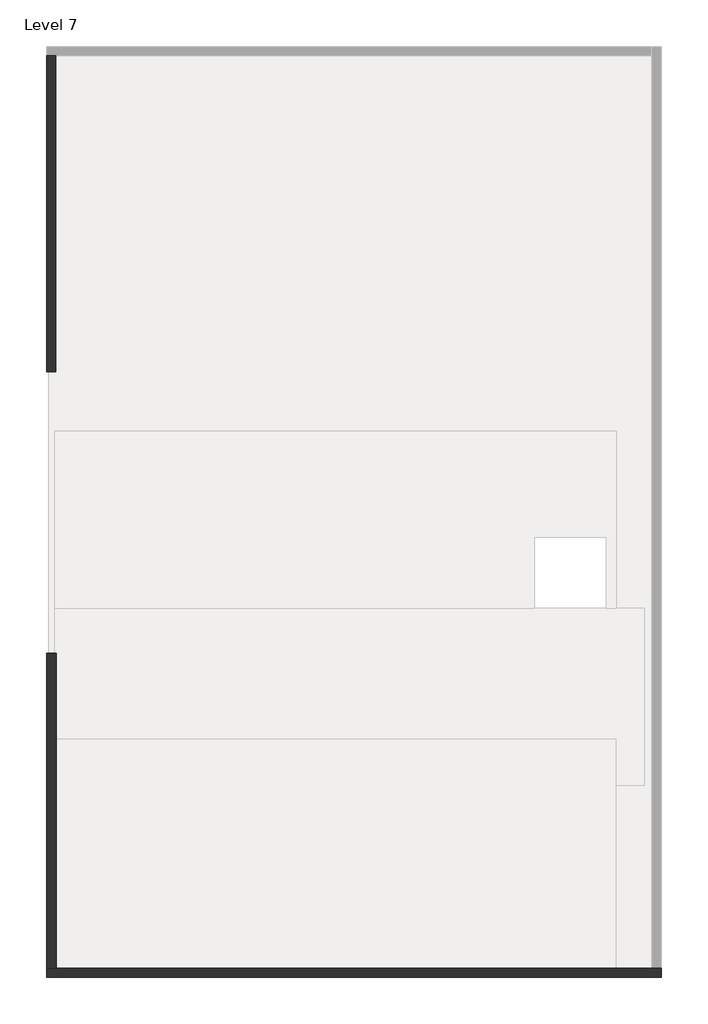
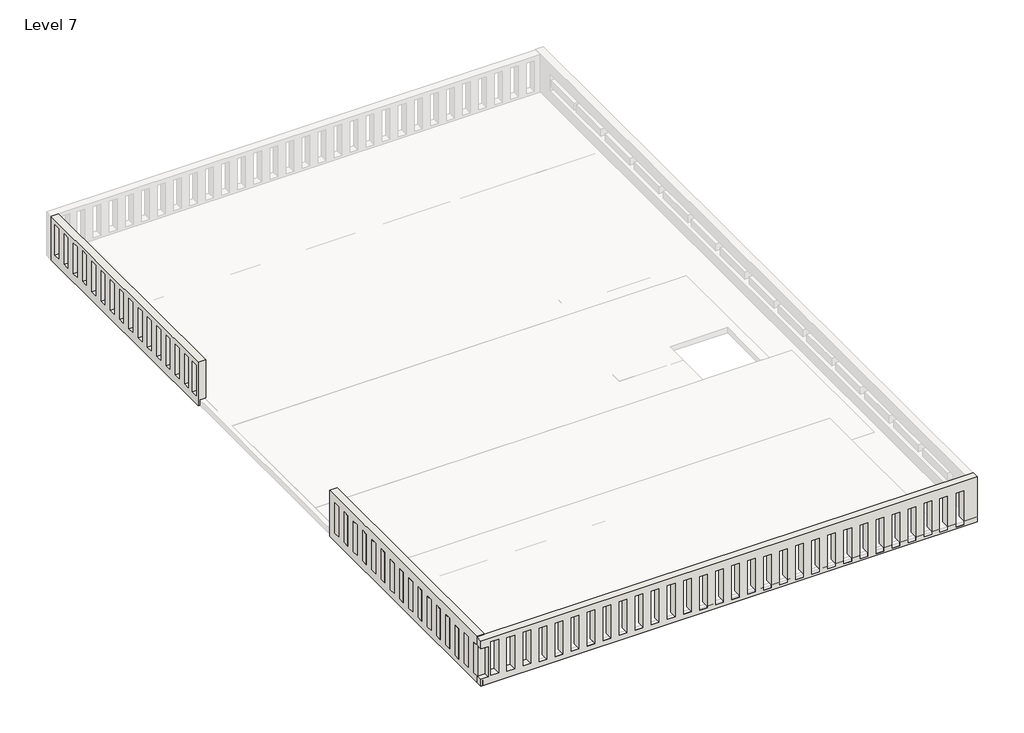
# One storey, part 1 of 2: 3 walls.
"""IFC4 building model written with IfcOpenShell, lengths in millimetres."""

from ifc_helpers import new_model, si_unit, origin, place, context, project, spatial, faceted_brep, element, save

model = new_model("IFC4")

# Units and contexts
model_context = context("Model", 3, world=origin())
ifc_project = project(units=[si_unit("LENGTHUNIT", "METRE", prefix="MILLI")], contexts=[model_context])

# Site, building, storey
site = spatial("IfcSite", under=ifc_project)
building = spatial("IfcBuilding", under=site)
storey = spatial("IfcBuildingStorey", under=building, Name="Level 7", Elevation=18288.0)

# Walls
placement = place(None, origin())
element("IfcWall", 1, ObjectType="Generic - 9\" w", at=placement, inside=storey, context=model_context, shape_type="Brep", body=[
    faceted_brep([(6853.7890963, -10500.4694836, 18288.0), (6650.5890963, -10500.4694836, 18288.0), (-6296.5895774, -10500.4694836, 18288.0), (-6499.7895774, -10500.4694836, 18288.0), (-6499.7895774, -10500.4694836, 18487.795072), (-6303.4109037, -10500.4694836, 18487.795072), (-6303.4109037, -10500.4694836, 19351.395072), (-6499.7895774, -10500.4694836, 19351.395072), (-6499.7895774, -10500.4694836, 19568.7926921), (6853.7890963, -10500.4694836, 19568.7926921), (6853.7890963, -10500.4694836, 19542.6572919), (-6026.0013636, -10500.4694836, 19465.6802167), (-6229.2013636, -10500.4694836, 19465.6802167), (-6229.2013636, -10500.4694836, 18509.4623037), (-6026.0013636, -10500.4694836, 18509.4623037), (-5595.844493, -10500.4694836, 19428.046367), (-5799.044493, -10500.4694836, 19428.046367), (-5799.044493, -10500.4694836, 18471.8284539), (-5595.844493, -10500.4694836, 18471.8284539), (-5164.044493, -10500.4694836, 19428.046367), (-5367.244493, -10500.4694836, 19428.046367), (-5367.244493, -10500.4694836, 18471.8284539), (-5164.044493, -10500.4694836, 18471.8284539), (-4733.8876223, -10500.4694836, 19390.4125173), (-4937.0876223, -10500.4694836, 19390.4125173), (-4937.0876223, -10500.4694836, 18434.1946042), (-4733.8876223, -10500.4694836, 18434.1946042), (-4302.0876223, -10500.4694836, 19390.4125173), (-4505.2876223, -10500.4694836, 19390.4125173), (-4505.2876223, -10500.4694836, 18434.1946042), (-4302.0876223, -10500.4694836, 18434.1946042), (-3870.2876223, -10500.4694836, 19390.4125173), (-4073.4876223, -10500.4694836, 19390.4125173), (-4073.4876223, -10500.4694836, 18434.1946042), (-3870.2876223, -10500.4694836, 18434.1946042), (-3438.4876223, -10500.4694836, 19390.4125173), (-3641.6876223, -10500.4694836, 19390.4125173), (-3641.6876223, -10500.4694836, 18434.1946042), (-3438.4876223, -10500.4694836, 18434.1946042), (-3006.6876223, -10500.4694836, 19390.4125173), (-3209.8876223, -10500.4694836, 19390.4125173), (-3209.8876223, -10500.4694836, 18434.1946042), (-3006.6876223, -10500.4694836, 18434.1946042), (-2574.8876223, -10500.4694836, 19390.4125173), (-2778.0876223, -10500.4694836, 19390.4125173), (-2778.0876223, -10500.4694836, 18434.1946042), (-2574.8876223, -10500.4694836, 18434.1946042), (-2143.0876223, -10500.4694836, 19390.4125173), (-2346.2876223, -10500.4694836, 19390.4125173), (-2346.2876223, -10500.4694836, 18434.1946042), (-2143.0876223, -10500.4694836, 18434.1946042), (-1711.2876223, -10500.4694836, 19390.4125173), (-1914.4876223, -10500.4694836, 19390.4125173), (-1914.4876223, -10500.4694836, 18434.1946042), (-1711.2876223, -10500.4694836, 18434.1946042), (-1279.4876223, -10500.4694836, 19390.4125173), (-1482.6876223, -10500.4694836, 19390.4125173), (-1482.6876223, -10500.4694836, 18434.1946042), (-1279.4876223, -10500.4694836, 18434.1946042), (-847.6876223, -10500.4694836, 19390.4125173), (-1050.8876223, -10500.4694836, 19390.4125173), (-1050.8876223, -10500.4694836, 18434.1946042), (-847.6876223, -10500.4694836, 18434.1946042), (-417.5307517, -10500.4694836, 19352.7786675), (-620.7307517, -10500.4694836, 19352.7786675), (-620.7307517, -10500.4694836, 18396.5607545), (-417.5307517, -10500.4694836, 18396.5607545), (14.2692483, -10500.4694836, 19352.7786675), (-188.9307517, -10500.4694836, 19352.7786675), (-188.9307517, -10500.4694836, 18396.5607545), (14.2692483, -10500.4694836, 18396.5607545), (446.0692483, -10500.4694836, 19352.7786675), (242.8692483, -10500.4694836, 19352.7786675), (242.8692483, -10500.4694836, 18396.5607545), (446.0692483, -10500.4694836, 18396.5607545), (877.8692483, -10500.4694836, 19352.7786675), (674.6692483, -10500.4694836, 19352.7786675), (674.6692483, -10500.4694836, 18396.5607545), (877.8692483, -10500.4694836, 18396.5607545), (1308.0261189, -10500.4694836, 19315.1448178), (1104.8261189, -10500.4694836, 19315.1448178), (1104.8261189, -10500.4694836, 18358.9269048), (1308.0261189, -10500.4694836, 18358.9269048), (1739.8261189, -10500.4694836, 19315.1448178), (1536.6261189, -10500.4694836, 19315.1448178), (1536.6261189, -10500.4694836, 18358.9269048), (1739.8261189, -10500.4694836, 18358.9269048), (2171.6261189, -10500.4694836, 19315.1448178), (1968.4261189, -10500.4694836, 19315.1448178), (1968.4261189, -10500.4694836, 18358.9269048), (2171.6261189, -10500.4694836, 18358.9269048), (2603.4261189, -10500.4694836, 19315.1448178), (2400.2261189, -10500.4694836, 19315.1448178), (2400.2261189, -10500.4694836, 18358.9269048), (2603.4261189, -10500.4694836, 18358.9269048), (3035.2261189, -10500.4694836, 19315.1448178), (2832.0261189, -10500.4694836, 19315.1448178), (2832.0261189, -10500.4694836, 18358.9269048), (3035.2261189, -10500.4694836, 18358.9269048), (3467.0261189, -10500.4694836, 19315.1448178), (3263.8261189, -10500.4694836, 19315.1448178), (3263.8261189, -10500.4694836, 18358.9269048), (3467.0261189, -10500.4694836, 18358.9269048), (3898.5630781, -10500.4694836, 19300.0752152), (3695.3630781, -10500.4694836, 19300.0752152), (3695.3630781, -10500.4694836, 18343.8573021), (3898.5630781, -10500.4694836, 18343.8573021), (4330.3630781, -10500.4694836, 19300.0752152), (4127.1630781, -10500.4694836, 19300.0752152), (4127.1630781, -10500.4694836, 18343.8573021), (4330.3630781, -10500.4694836, 18343.8573021), (4762.1630781, -10500.4694836, 19300.0752152), (4558.9630781, -10500.4694836, 19300.0752152), (4558.9630781, -10500.4694836, 18343.8573021), (4762.1630781, -10500.4694836, 18343.8573021), (5193.9630781, -10500.4694836, 19300.0752152), (4990.7630781, -10500.4694836, 19300.0752152), (4990.7630781, -10500.4694836, 18343.8573021), (5193.9630781, -10500.4694836, 18343.8573021), (6044.4430536, -10500.4694836, 19300.0752152), (5841.2430536, -10500.4694836, 19300.0752152), (5841.2430536, -10500.4694836, 18343.8573021), (6044.4430536, -10500.4694836, 18343.8573021), (6485.4890963, -10500.4694836, 19300.0752152), (6282.2890963, -10500.4694836, 19300.0752152), (6282.2890963, -10500.4694836, 18343.8573021), (6485.4890963, -10500.4694836, 18343.8573021), (5625.1713112, -10500.4694836, 19322.6738811), (5421.9713112, -10500.4694836, 19322.6738811), (5421.9713112, -10500.4694836, 18366.455968), (5625.1713112, -10500.4694836, 18366.455968), (6853.7890963, -10703.6694836, 18288.0), (6853.7890963, -10703.6694836, 19568.7926921), (-6499.7895774, -10703.6694836, 19568.7926921), (-6499.7895774, -10703.6694836, 19351.395072), (-6303.4109037, -10703.6694836, 19351.395072), (-6303.4109037, -10703.6694836, 18487.795072), (-6499.7895774, -10703.6694836, 18487.795072), (-6499.7895774, -10703.6694836, 18288.0), (-6026.0013636, -10703.6694836, 19465.6802167), (-6026.0013636, -10703.6694836, 18509.4623037), (-6229.2013636, -10703.6694836, 18509.4623037), (-6229.2013636, -10703.6694836, 19465.6802167), (-5595.844493, -10703.6694836, 19428.046367), (-5595.844493, -10703.6694836, 18471.8284539), (-5799.044493, -10703.6694836, 18471.8284539), (-5799.044493, -10703.6694836, 19428.046367), (-5164.044493, -10703.6694836, 19428.046367), (-5164.044493, -10703.6694836, 18471.8284539), (-5367.244493, -10703.6694836, 18471.8284539), (-5367.244493, -10703.6694836, 19428.046367), (-4733.8876223, -10703.6694836, 19390.4125173), (-4733.8876223, -10703.6694836, 18434.1946042), (-4937.0876223, -10703.6694836, 18434.1946042), (-4937.0876223, -10703.6694836, 19390.4125173), (-4302.0876223, -10703.6694836, 19390.4125173), (-4302.0876223, -10703.6694836, 18434.1946042), (-4505.2876223, -10703.6694836, 18434.1946042), (-4505.2876223, -10703.6694836, 19390.4125173), (-3870.2876223, -10703.6694836, 19390.4125173), (-3870.2876223, -10703.6694836, 18434.1946042), (-4073.4876223, -10703.6694836, 18434.1946042), (-4073.4876223, -10703.6694836, 19390.4125173), (-3438.4876223, -10703.6694836, 19390.4125173), (-3438.4876223, -10703.6694836, 18434.1946042), (-3641.6876223, -10703.6694836, 18434.1946042), (-3641.6876223, -10703.6694836, 19390.4125173), (-3006.6876223, -10703.6694836, 19390.4125173), (-3006.6876223, -10703.6694836, 18434.1946042), (-3209.8876223, -10703.6694836, 18434.1946042), (-3209.8876223, -10703.6694836, 19390.4125173), (-2574.8876223, -10703.6694836, 19390.4125173), (-2574.8876223, -10703.6694836, 18434.1946042), (-2778.0876223, -10703.6694836, 18434.1946042), (-2778.0876223, -10703.6694836, 19390.4125173), (-2143.0876223, -10703.6694836, 19390.4125173), (-2143.0876223, -10703.6694836, 18434.1946042), (-2346.2876223, -10703.6694836, 18434.1946042), (-2346.2876223, -10703.6694836, 19390.4125173), (-1711.2876223, -10703.6694836, 19390.4125173), (-1711.2876223, -10703.6694836, 18434.1946042), (-1914.4876223, -10703.6694836, 18434.1946042), (-1914.4876223, -10703.6694836, 19390.4125173), (-1279.4876223, -10703.6694836, 19390.4125173), (-1279.4876223, -10703.6694836, 18434.1946042), (-1482.6876223, -10703.6694836, 18434.1946042), (-1482.6876223, -10703.6694836, 19390.4125173), (-847.6876223, -10703.6694836, 19390.4125173), (-847.6876223, -10703.6694836, 18434.1946042), (-1050.8876223, -10703.6694836, 18434.1946042), (-1050.8876223, -10703.6694836, 19390.4125173), (-417.5307517, -10703.6694836, 19352.7786675), (-417.5307517, -10703.6694836, 18396.5607545), (-620.7307517, -10703.6694836, 18396.5607545), (-620.7307517, -10703.6694836, 19352.7786675), (14.2692483, -10703.6694836, 19352.7786675), (14.2692483, -10703.6694836, 18396.5607545), (-188.9307517, -10703.6694836, 18396.5607545), (-188.9307517, -10703.6694836, 19352.7786675), (446.0692483, -10703.6694836, 19352.7786675), (446.0692483, -10703.6694836, 18396.5607545), (242.8692483, -10703.6694836, 18396.5607545), (242.8692483, -10703.6694836, 19352.7786675), (877.8692483, -10703.6694836, 19352.7786675), (877.8692483, -10703.6694836, 18396.5607545), (674.6692483, -10703.6694836, 18396.5607545), (674.6692483, -10703.6694836, 19352.7786675), (1308.0261189, -10703.6694836, 19315.1448178), (1308.0261189, -10703.6694836, 18358.9269048), (1104.8261189, -10703.6694836, 18358.9269048), (1104.8261189, -10703.6694836, 19315.1448178), (1739.8261189, -10703.6694836, 19315.1448178), (1739.8261189, -10703.6694836, 18358.9269048), (1536.6261189, -10703.6694836, 18358.9269048), (1536.6261189, -10703.6694836, 19315.1448178), (2171.6261189, -10703.6694836, 19315.1448178), (2171.6261189, -10703.6694836, 18358.9269048), (1968.4261189, -10703.6694836, 18358.9269048), (1968.4261189, -10703.6694836, 19315.1448178), (2603.4261189, -10703.6694836, 19315.1448178), (2603.4261189, -10703.6694836, 18358.9269048), (2400.2261189, -10703.6694836, 18358.9269048), (2400.2261189, -10703.6694836, 19315.1448178), (3035.2261189, -10703.6694836, 19315.1448178), (3035.2261189, -10703.6694836, 18358.9269048), (2832.0261189, -10703.6694836, 18358.9269048), (2832.0261189, -10703.6694836, 19315.1448178), (3467.0261189, -10703.6694836, 19315.1448178), (3467.0261189, -10703.6694836, 18358.9269048), (3263.8261189, -10703.6694836, 18358.9269048), (3263.8261189, -10703.6694836, 19315.1448178), (3898.5630781, -10703.6694836, 19300.0752152), (3898.5630781, -10703.6694836, 18343.8573021), (3695.3630781, -10703.6694836, 18343.8573021), (3695.3630781, -10703.6694836, 19300.0752152), (4330.3630781, -10703.6694836, 19300.0752152), (4330.3630781, -10703.6694836, 18343.8573021), (4127.1630781, -10703.6694836, 18343.8573021), (4127.1630781, -10703.6694836, 19300.0752152), (4762.1630781, -10703.6694836, 19300.0752152), (4762.1630781, -10703.6694836, 18343.8573021), (4558.9630781, -10703.6694836, 18343.8573021), (4558.9630781, -10703.6694836, 19300.0752152), (5193.9630781, -10703.6694836, 19300.0752152), (5193.9630781, -10703.6694836, 18343.8573021), (4990.7630781, -10703.6694836, 18343.8573021), (4990.7630781, -10703.6694836, 19300.0752152), (6044.4430536, -10703.6694836, 19300.0752152), (6044.4430536, -10703.6694836, 18343.8573021), (5841.2430536, -10703.6694836, 18343.8573021), (5841.2430536, -10703.6694836, 19300.0752152), (6485.4890963, -10703.6694836, 19300.0752152), (6485.4890963, -10703.6694836, 18343.8573021), (6282.2890963, -10703.6694836, 18343.8573021), (6282.2890963, -10703.6694836, 19300.0752152), (5625.1713112, -10703.6694836, 19322.6738811), (5625.1713112, -10703.6694836, 18366.455968), (5421.9713112, -10703.6694836, 18366.455968), (5421.9713112, -10703.6694836, 19322.6738811), (-6303.4109037, -10557.1743868, 18487.795072), (-6303.4109037, -10557.1743868, 19351.395072)], [[[0, 1, 2, 3, 4, 5, 6, 7, 8, 9, 10], [11, 12, 13, 14], [15, 16, 17, 18], [19, 20, 21, 22], [23, 24, 25, 26], [27, 28, 29, 30], [31, 32, 33, 34], [35, 36, 37, 38], [39, 40, 41, 42], [43, 44, 45, 46], [47, 48, 49, 50], [51, 52, 53, 54], [55, 56, 57, 58], [59, 60, 61, 62], [63, 64, 65, 66], [67, 68, 69, 70], [71, 72, 73, 74], [75, 76, 77, 78], [79, 80, 81, 82], [83, 84, 85, 86], [87, 88, 89, 90], [91, 92, 93, 94], [95, 96, 97, 98], [99, 100, 101, 102], [103, 104, 105, 106], [107, 108, 109, 110], [111, 112, 113, 114], [115, 116, 117, 118], [119, 120, 121, 122], [123, 124, 125, 126], [127, 128, 129, 130]], [[131, 132, 133, 134, 135, 136, 137, 138], [139, 140, 141, 142], [143, 144, 145, 146], [147, 148, 149, 150], [151, 152, 153, 154], [155, 156, 157, 158], [159, 160, 161, 162], [163, 164, 165, 166], [167, 168, 169, 170], [171, 172, 173, 174], [175, 176, 177, 178], [179, 180, 181, 182], [183, 184, 185, 186], [187, 188, 189, 190], [191, 192, 193, 194], [195, 196, 197, 198], [199, 200, 201, 202], [203, 204, 205, 206], [207, 208, 209, 210], [211, 212, 213, 214], [215, 216, 217, 218], [219, 220, 221, 222], [223, 224, 225, 226], [227, 228, 229, 230], [231, 232, 233, 234], [235, 236, 237, 238], [239, 240, 241, 242], [243, 244, 245, 246], [247, 248, 249, 250], [251, 252, 253, 254], [255, 256, 257, 258]], [[0, 10, 9, 132, 131]], [[4, 3, 138, 137]], [[6, 5, 259, 136, 135, 260]], [[8, 7, 134, 133]], [[3, 2, 1, 0, 131, 138]], [[9, 8, 133, 132]], [[136, 259, 5, 4, 137]], [[134, 7, 6, 260, 135]], [[12, 11, 139, 142]], [[13, 12, 142, 141]], [[14, 13, 141, 140]], [[11, 14, 140, 139]], [[16, 15, 143, 146]], [[17, 16, 146, 145]], [[18, 17, 145, 144]], [[15, 18, 144, 143]], [[20, 19, 147, 150]], [[21, 20, 150, 149]], [[22, 21, 149, 148]], [[19, 22, 148, 147]], [[24, 23, 151, 154]], [[25, 24, 154, 153]], [[26, 25, 153, 152]], [[23, 26, 152, 151]], [[28, 27, 155, 158]], [[29, 28, 158, 157]], [[30, 29, 157, 156]], [[27, 30, 156, 155]], [[32, 31, 159, 162]], [[33, 32, 162, 161]], [[34, 33, 161, 160]], [[31, 34, 160, 159]], [[36, 35, 163, 166]], [[37, 36, 166, 165]], [[38, 37, 165, 164]], [[35, 38, 164, 163]], [[40, 39, 167, 170]], [[41, 40, 170, 169]], [[42, 41, 169, 168]], [[39, 42, 168, 167]], [[44, 43, 171, 174]], [[45, 44, 174, 173]], [[46, 45, 173, 172]], [[43, 46, 172, 171]], [[48, 47, 175, 178]], [[49, 48, 178, 177]], [[50, 49, 177, 176]], [[47, 50, 176, 175]], [[52, 51, 179, 182]], [[53, 52, 182, 181]], [[54, 53, 181, 180]], [[51, 54, 180, 179]], [[56, 55, 183, 186]], [[57, 56, 186, 185]], [[58, 57, 185, 184]], [[55, 58, 184, 183]], [[60, 59, 187, 190]], [[61, 60, 190, 189]], [[62, 61, 189, 188]], [[59, 62, 188, 187]], [[64, 63, 191, 194]], [[65, 64, 194, 193]], [[66, 65, 193, 192]], [[63, 66, 192, 191]], [[68, 67, 195, 198]], [[69, 68, 198, 197]], [[70, 69, 197, 196]], [[67, 70, 196, 195]], [[72, 71, 199, 202]], [[73, 72, 202, 201]], [[74, 73, 201, 200]], [[71, 74, 200, 199]], [[76, 75, 203, 206]], [[77, 76, 206, 205]], [[78, 77, 205, 204]], [[75, 78, 204, 203]], [[80, 79, 207, 210]], [[81, 80, 210, 209]], [[82, 81, 209, 208]], [[79, 82, 208, 207]], [[84, 83, 211, 214]], [[85, 84, 214, 213]], [[86, 85, 213, 212]], [[83, 86, 212, 211]], [[88, 87, 215, 218]], [[89, 88, 218, 217]], [[90, 89, 217, 216]], [[87, 90, 216, 215]], [[92, 91, 219, 222]], [[93, 92, 222, 221]], [[94, 93, 221, 220]], [[91, 94, 220, 219]], [[96, 95, 223, 226]], [[97, 96, 226, 225]], [[98, 97, 225, 224]], [[95, 98, 224, 223]], [[100, 99, 227, 230]], [[101, 100, 230, 229]], [[102, 101, 229, 228]], [[99, 102, 228, 227]], [[104, 103, 231, 234]], [[105, 104, 234, 233]], [[106, 105, 233, 232]], [[103, 106, 232, 231]], [[108, 107, 235, 238]], [[109, 108, 238, 237]], [[110, 109, 237, 236]], [[107, 110, 236, 235]], [[112, 111, 239, 242]], [[113, 112, 242, 241]], [[114, 113, 241, 240]], [[111, 114, 240, 239]], [[116, 115, 243, 246]], [[117, 116, 246, 245]], [[118, 117, 245, 244]], [[115, 118, 244, 243]], [[120, 119, 247, 250]], [[121, 120, 250, 249]], [[122, 121, 249, 248]], [[119, 122, 248, 247]], [[124, 123, 251, 254]], [[125, 124, 254, 253]], [[126, 125, 253, 252]], [[123, 126, 252, 251]], [[128, 127, 255, 258]], [[129, 128, 258, 257]], [[130, 129, 257, 256]], [[127, 130, 256, 255]]]),
])
element("IfcWall", 2, ObjectType="Generic - 9\" w", at=placement, inside=storey, context=model_context, shape_type="Brep", body=[
    faceted_brep([(-6506.6109037, 9313.3962251, 18288.0), (-6506.6109037, 2455.3962251, 18288.0), (-6506.6109037, 2455.3962251, 19520.2498043), (-6506.6109037, 9313.3962251, 19520.2498043), (-6506.6109037, 8952.0816143, 19389.0289217), (-6506.6109037, 8952.0816143, 18525.4289217), (-6506.6109037, 9129.8816143, 18525.4289217), (-6506.6109037, 9129.8816143, 19389.0289217), (-6506.6109037, 8520.2816143, 19389.0289217), (-6506.6109037, 8520.2816143, 18525.4289217), (-6506.6109037, 8698.0816143, 18525.4289217), (-6506.6109037, 8698.0816143, 19389.0289217), (-6506.6109037, 8088.4816143, 19389.0289217), (-6506.6109037, 8088.4816143, 18525.4289217), (-6506.6109037, 8266.2816143, 18525.4289217), (-6506.6109037, 8266.2816143, 19389.0289217), (-6506.6109037, 7658.3247436, 19426.6627714), (-6506.6109037, 7658.3247436, 18563.0627714), (-6506.6109037, 7836.1247436, 18563.0627714), (-6506.6109037, 7836.1247436, 19426.6627714), (-6506.6109037, 7228.167873, 19389.0289217), (-6506.6109037, 7228.167873, 18525.4289217), (-6506.6109037, 7405.967873, 18525.4289217), (-6506.6109037, 7405.967873, 19389.0289217), (-6506.6109037, 6796.367873, 19389.0289217), (-6506.6109037, 6796.367873, 18525.4289217), (-6506.6109037, 6974.167873, 18525.4289217), (-6506.6109037, 6974.167873, 19389.0289217), (-6506.6109037, 6364.567873, 19389.0289217), (-6506.6109037, 6364.567873, 18525.4289217), (-6506.6109037, 6542.367873, 18525.4289217), (-6506.6109037, 6542.367873, 19389.0289217), (-6506.6109037, 5932.767873, 19389.0289217), (-6506.6109037, 5932.767873, 18525.4289217), (-6506.6109037, 6110.567873, 18525.4289217), (-6506.6109037, 6110.567873, 19389.0289217), (-6506.6109037, 5500.967873, 19389.0289217), (-6506.6109037, 5500.967873, 18525.4289217), (-6506.6109037, 5678.767873, 18525.4289217), (-6506.6109037, 5678.767873, 19389.0289217), (-6506.6109037, 5069.167873, 19389.0289217), (-6506.6109037, 5069.167873, 18525.4289217), (-6506.6109037, 5246.967873, 18525.4289217), (-6506.6109037, 5246.967873, 19389.0289217), (-6506.6109037, 4637.367873, 19389.0289217), (-6506.6109037, 4637.367873, 18525.4289217), (-6506.6109037, 4815.167873, 18525.4289217), (-6506.6109037, 4815.167873, 19389.0289217), (-6506.6109037, 4205.567873, 19389.0289217), (-6506.6109037, 4205.567873, 18525.4289217), (-6506.6109037, 4383.367873, 18525.4289217), (-6506.6109037, 4383.367873, 19389.0289217), (-6506.6109037, 3773.767873, 19389.0289217), (-6506.6109037, 3773.767873, 18525.4289217), (-6506.6109037, 3951.567873, 18525.4289217), (-6506.6109037, 3951.567873, 19389.0289217), (-6506.6109037, 3341.967873, 19389.0289217), (-6506.6109037, 3341.967873, 18525.4289217), (-6506.6109037, 3519.767873, 18525.4289217), (-6506.6109037, 3519.767873, 19389.0289217), (-6506.6109037, 2910.167873, 19389.0289217), (-6506.6109037, 2910.167873, 18525.4289217), (-6506.6109037, 3087.967873, 18525.4289217), (-6506.6109037, 3087.967873, 19389.0289217), (-6506.6109037, 2544.2962251, 19389.0289217), (-6506.6109037, 2544.2962251, 18525.4289217), (-6506.6109037, 2722.0962251, 18525.4289217), (-6506.6109037, 2722.0962251, 19389.0289217), (-6303.4109037, 9313.3962251, 18288.0), (-6303.4109037, 9313.3962251, 19520.2498043), (-6303.4109037, 2455.3962251, 19520.2498043), (-6303.4109037, 2455.3962251, 18288.0), (-6303.4109037, 8952.0816143, 19389.0289217), (-6303.4109037, 9129.8816143, 19389.0289217), (-6303.4109037, 9129.8816143, 18525.4289217), (-6303.4109037, 8952.0816143, 18525.4289217), (-6303.4109037, 8520.2816143, 19389.0289217), (-6303.4109037, 8698.0816143, 19389.0289217), (-6303.4109037, 8698.0816143, 18525.4289217), (-6303.4109037, 8520.2816143, 18525.4289217), (-6303.4109037, 8088.4816143, 19389.0289217), (-6303.4109037, 8266.2816143, 19389.0289217), (-6303.4109037, 8266.2816143, 18525.4289217), (-6303.4109037, 8088.4816143, 18525.4289217), (-6303.4109037, 7658.3247436, 19426.6627714), (-6303.4109037, 7836.1247436, 19426.6627714), (-6303.4109037, 7836.1247436, 18563.0627714), (-6303.4109037, 7658.3247436, 18563.0627714), (-6303.4109037, 7228.167873, 19389.0289217), (-6303.4109037, 7405.967873, 19389.0289217), (-6303.4109037, 7405.967873, 18525.4289217), (-6303.4109037, 7228.167873, 18525.4289217), (-6303.4109037, 6796.367873, 19389.0289217), (-6303.4109037, 6974.167873, 19389.0289217), (-6303.4109037, 6974.167873, 18525.4289217), (-6303.4109037, 6796.367873, 18525.4289217), (-6303.4109037, 6364.567873, 19389.0289217), (-6303.4109037, 6542.367873, 19389.0289217), (-6303.4109037, 6542.367873, 18525.4289217), (-6303.4109037, 6364.567873, 18525.4289217), (-6303.4109037, 5932.767873, 19389.0289217), (-6303.4109037, 6110.567873, 19389.0289217), (-6303.4109037, 6110.567873, 18525.4289217), (-6303.4109037, 5932.767873, 18525.4289217), (-6303.4109037, 5500.967873, 19389.0289217), (-6303.4109037, 5678.767873, 19389.0289217), (-6303.4109037, 5678.767873, 18525.4289217), (-6303.4109037, 5500.967873, 18525.4289217), (-6303.4109037, 5069.167873, 19389.0289217), (-6303.4109037, 5246.967873, 19389.0289217), (-6303.4109037, 5246.967873, 18525.4289217), (-6303.4109037, 5069.167873, 18525.4289217), (-6303.4109037, 4637.367873, 19389.0289217), (-6303.4109037, 4815.167873, 19389.0289217), (-6303.4109037, 4815.167873, 18525.4289217), (-6303.4109037, 4637.367873, 18525.4289217), (-6303.4109037, 4205.567873, 19389.0289217), (-6303.4109037, 4383.367873, 19389.0289217), (-6303.4109037, 4383.367873, 18525.4289217), (-6303.4109037, 4205.567873, 18525.4289217), (-6303.4109037, 3773.767873, 19389.0289217), (-6303.4109037, 3951.567873, 19389.0289217), (-6303.4109037, 3951.567873, 18525.4289217), (-6303.4109037, 3773.767873, 18525.4289217), (-6303.4109037, 3341.967873, 19389.0289217), (-6303.4109037, 3519.767873, 19389.0289217), (-6303.4109037, 3519.767873, 18525.4289217), (-6303.4109037, 3341.967873, 18525.4289217), (-6303.4109037, 2910.167873, 19389.0289217), (-6303.4109037, 3087.967873, 19389.0289217), (-6303.4109037, 3087.967873, 18525.4289217), (-6303.4109037, 2910.167873, 18525.4289217), (-6303.4109037, 2544.2962251, 19389.0289217), (-6303.4109037, 2722.0962251, 19389.0289217), (-6303.4109037, 2722.0962251, 18525.4289217), (-6303.4109037, 2544.2962251, 18525.4289217)], [[[0, 1, 2, 3], [4, 5, 6, 7], [8, 9, 10, 11], [12, 13, 14, 15], [16, 17, 18, 19], [20, 21, 22, 23], [24, 25, 26, 27], [28, 29, 30, 31], [32, 33, 34, 35], [36, 37, 38, 39], [40, 41, 42, 43], [44, 45, 46, 47], [48, 49, 50, 51], [52, 53, 54, 55], [56, 57, 58, 59], [60, 61, 62, 63], [64, 65, 66, 67]], [[68, 69, 70, 71], [72, 73, 74, 75], [76, 77, 78, 79], [80, 81, 82, 83], [84, 85, 86, 87], [88, 89, 90, 91], [92, 93, 94, 95], [96, 97, 98, 99], [100, 101, 102, 103], [104, 105, 106, 107], [108, 109, 110, 111], [112, 113, 114, 115], [116, 117, 118, 119], [120, 121, 122, 123], [124, 125, 126, 127], [128, 129, 130, 131], [132, 133, 134, 135]], [[0, 3, 69, 68]], [[1, 0, 68, 71]], [[2, 1, 71, 70]], [[3, 2, 70, 69]], [[5, 4, 72, 75]], [[6, 5, 75, 74]], [[7, 6, 74, 73]], [[4, 7, 73, 72]], [[9, 8, 76, 79]], [[10, 9, 79, 78]], [[11, 10, 78, 77]], [[8, 11, 77, 76]], [[13, 12, 80, 83]], [[14, 13, 83, 82]], [[15, 14, 82, 81]], [[12, 15, 81, 80]], [[17, 16, 84, 87]], [[18, 17, 87, 86]], [[19, 18, 86, 85]], [[16, 19, 85, 84]], [[21, 20, 88, 91]], [[22, 21, 91, 90]], [[23, 22, 90, 89]], [[20, 23, 89, 88]], [[25, 24, 92, 95]], [[26, 25, 95, 94]], [[27, 26, 94, 93]], [[24, 27, 93, 92]], [[29, 28, 96, 99]], [[30, 29, 99, 98]], [[31, 30, 98, 97]], [[28, 31, 97, 96]], [[33, 32, 100, 103]], [[34, 33, 103, 102]], [[35, 34, 102, 101]], [[32, 35, 101, 100]], [[37, 36, 104, 107]], [[38, 37, 107, 106]], [[39, 38, 106, 105]], [[36, 39, 105, 104]], [[41, 40, 108, 111]], [[42, 41, 111, 110]], [[43, 42, 110, 109]], [[40, 43, 109, 108]], [[45, 44, 112, 115]], [[46, 45, 115, 114]], [[47, 46, 114, 113]], [[44, 47, 113, 112]], [[49, 48, 116, 119]], [[50, 49, 119, 118]], [[51, 50, 118, 117]], [[48, 51, 117, 116]], [[53, 52, 120, 123]], [[54, 53, 123, 122]], [[55, 54, 122, 121]], [[52, 55, 121, 120]], [[57, 56, 124, 127]], [[58, 57, 127, 126]], [[59, 58, 126, 125]], [[56, 59, 125, 124]], [[61, 60, 128, 131]], [[62, 61, 131, 130]], [[63, 62, 130, 129]], [[60, 63, 129, 128]], [[65, 64, 132, 135]], [[66, 65, 135, 134]], [[67, 66, 134, 133]], [[64, 67, 133, 132]]]),
    faceted_brep([(-6506.6109037, -4085.1037749, 19389.0289217), (-6506.6109037, -3907.3037749, 19389.0289217), (-6506.6109037, -3907.3037749, 18525.4289217), (-6506.6109037, -4085.1037749, 18525.4289217), (-6303.4109037, -4085.1037749, 19389.0289217), (-6303.4109037, -4085.1037749, 18525.4289217), (-6303.4109037, -3907.3037749, 18525.4289217), (-6303.4109037, -3907.3037749, 19389.0289217)], [[[0, 1, 2, 3]], [[4, 5, 6, 7]], [[1, 0, 4, 7]], [[2, 1, 7, 6]], [[3, 2, 6, 5]], [[0, 3, 5, 4]]]),
    faceted_brep([(-6506.6109037, -4516.9037749, 19389.0289217), (-6506.6109037, -4339.1037749, 19389.0289217), (-6506.6109037, -4339.1037749, 18525.4289217), (-6506.6109037, -4516.9037749, 18525.4289217), (-6303.4109037, -4516.9037749, 19389.0289217), (-6303.4109037, -4516.9037749, 18525.4289217), (-6303.4109037, -4339.1037749, 18525.4289217), (-6303.4109037, -4339.1037749, 19389.0289217)], [[[0, 1, 2, 3]], [[4, 5, 6, 7]], [[1, 0, 4, 7]], [[2, 1, 7, 6]], [[3, 2, 6, 5]], [[0, 3, 5, 4]]]),
    faceted_brep([(-6506.6109037, -4948.7037749, 19389.0289217), (-6506.6109037, -4770.9037749, 19389.0289217), (-6506.6109037, -4770.9037749, 18525.4289217), (-6506.6109037, -4948.7037749, 18525.4289217), (-6303.4109037, -4948.7037749, 19389.0289217), (-6303.4109037, -4948.7037749, 18525.4289217), (-6303.4109037, -4770.9037749, 18525.4289217), (-6303.4109037, -4770.9037749, 19389.0289217)], [[[0, 1, 2, 3]], [[4, 5, 6, 7]], [[1, 0, 4, 7]], [[2, 1, 7, 6]], [[3, 2, 6, 5]], [[0, 3, 5, 4]]]),
    faceted_brep([(-6506.6109037, -5380.5037749, 19389.0289217), (-6506.6109037, -5202.7037749, 19389.0289217), (-6506.6109037, -5202.7037749, 18525.4289217), (-6506.6109037, -5380.5037749, 18525.4289217), (-6303.4109037, -5380.5037749, 19389.0289217), (-6303.4109037, -5380.5037749, 18525.4289217), (-6303.4109037, -5202.7037749, 18525.4289217), (-6303.4109037, -5202.7037749, 19389.0289217)], [[[0, 1, 2, 3]], [[4, 5, 6, 7]], [[1, 0, 4, 7]], [[2, 1, 7, 6]], [[3, 2, 6, 5]], [[0, 3, 5, 4]]]),
    faceted_brep([(-6506.6109037, -5812.3037749, 19389.0289217), (-6506.6109037, -5634.5037749, 19389.0289217), (-6506.6109037, -5634.5037749, 18525.4289217), (-6506.6109037, -5812.3037749, 18525.4289217), (-6303.4109037, -5812.3037749, 19389.0289217), (-6303.4109037, -5812.3037749, 18525.4289217), (-6303.4109037, -5634.5037749, 18525.4289217), (-6303.4109037, -5634.5037749, 19389.0289217)], [[[0, 1, 2, 3]], [[4, 5, 6, 7]], [[1, 0, 4, 7]], [[2, 1, 7, 6]], [[3, 2, 6, 5]], [[0, 3, 5, 4]]]),
    faceted_brep([(-6506.6109037, -6244.1037749, 19389.0289217), (-6506.6109037, -6066.3037749, 19389.0289217), (-6506.6109037, -6066.3037749, 18525.4289217), (-6506.6109037, -6244.1037749, 18525.4289217), (-6303.4109037, -6244.1037749, 19389.0289217), (-6303.4109037, -6244.1037749, 18525.4289217), (-6303.4109037, -6066.3037749, 18525.4289217), (-6303.4109037, -6066.3037749, 19389.0289217)], [[[0, 1, 2, 3]], [[4, 5, 6, 7]], [[1, 0, 4, 7]], [[2, 1, 7, 6]], [[3, 2, 6, 5]], [[0, 3, 5, 4]]]),
    faceted_brep([(-6506.6109037, -6674.2606456, 19351.395072), (-6506.6109037, -6496.4606456, 19351.395072), (-6506.6109037, -6496.4606456, 18487.795072), (-6506.6109037, -6674.2606456, 18487.795072), (-6303.4109037, -6674.2606456, 19351.395072), (-6303.4109037, -6674.2606456, 18487.795072), (-6303.4109037, -6496.4606456, 18487.795072), (-6303.4109037, -6496.4606456, 19351.395072)], [[[0, 1, 2, 3]], [[4, 5, 6, 7]], [[1, 0, 4, 7]], [[2, 1, 7, 6]], [[3, 2, 6, 5]], [[0, 3, 5, 4]]]),
    faceted_brep([(-6506.6109037, -7106.0606456, 19351.395072), (-6506.6109037, -6928.2606456, 19351.395072), (-6506.6109037, -6928.2606456, 18487.795072), (-6506.6109037, -7106.0606456, 18487.795072), (-6303.4109037, -7106.0606456, 19351.395072), (-6303.4109037, -7106.0606456, 18487.795072), (-6303.4109037, -6928.2606456, 18487.795072), (-6303.4109037, -6928.2606456, 19351.395072)], [[[0, 1, 2, 3]], [[4, 5, 6, 7]], [[1, 0, 4, 7]], [[2, 1, 7, 6]], [[3, 2, 6, 5]], [[0, 3, 5, 4]]]),
    faceted_brep([(-6506.6109037, -7537.8606456, 19351.395072), (-6506.6109037, -7360.0606456, 19351.395072), (-6506.6109037, -7360.0606456, 18487.795072), (-6506.6109037, -7537.8606456, 18487.795072), (-6303.4109037, -7537.8606456, 19351.395072), (-6303.4109037, -7537.8606456, 18487.795072), (-6303.4109037, -7360.0606456, 18487.795072), (-6303.4109037, -7360.0606456, 19351.395072)], [[[0, 1, 2, 3]], [[4, 5, 6, 7]], [[1, 0, 4, 7]], [[2, 1, 7, 6]], [[3, 2, 6, 5]], [[0, 3, 5, 4]]]),
    faceted_brep([(-6506.6109037, -7969.6606456, 19351.395072), (-6506.6109037, -7791.8606456, 19351.395072), (-6506.6109037, -7791.8606456, 18487.795072), (-6506.6109037, -7969.6606456, 18487.795072), (-6303.4109037, -7969.6606456, 19351.395072), (-6303.4109037, -7969.6606456, 18487.795072), (-6303.4109037, -7791.8606456, 18487.795072), (-6303.4109037, -7791.8606456, 19351.395072)], [[[0, 1, 2, 3]], [[4, 5, 6, 7]], [[1, 0, 4, 7]], [[2, 1, 7, 6]], [[3, 2, 6, 5]], [[0, 3, 5, 4]]]),
    faceted_brep([(-6506.6109037, -8401.4606456, 19351.395072), (-6506.6109037, -8223.6606456, 19351.395072), (-6506.6109037, -8223.6606456, 18487.795072), (-6506.6109037, -8401.4606456, 18487.795072), (-6303.4109037, -8401.4606456, 19351.395072), (-6303.4109037, -8401.4606456, 18487.795072), (-6303.4109037, -8223.6606456, 18487.795072), (-6303.4109037, -8223.6606456, 19351.395072)], [[[0, 1, 2, 3]], [[4, 5, 6, 7]], [[1, 0, 4, 7]], [[2, 1, 7, 6]], [[3, 2, 6, 5]], [[0, 3, 5, 4]]]),
    faceted_brep([(-6506.6109037, -8833.2606456, 19351.395072), (-6506.6109037, -8655.4606456, 19351.395072), (-6506.6109037, -8655.4606456, 18487.795072), (-6506.6109037, -8833.2606456, 18487.795072), (-6303.4109037, -8833.2606456, 19351.395072), (-6303.4109037, -8833.2606456, 18487.795072), (-6303.4109037, -8655.4606456, 18487.795072), (-6303.4109037, -8655.4606456, 19351.395072)], [[[0, 1, 2, 3]], [[4, 5, 6, 7]], [[1, 0, 4, 7]], [[2, 1, 7, 6]], [[3, 2, 6, 5]], [[0, 3, 5, 4]]]),
    faceted_brep([(-6506.6109037, -9265.0606456, 19351.395072), (-6506.6109037, -9087.2606456, 19351.395072), (-6506.6109037, -9087.2606456, 18487.795072), (-6506.6109037, -9265.0606456, 18487.795072), (-6303.4109037, -9265.0606456, 19351.395072), (-6303.4109037, -9265.0606456, 18487.795072), (-6303.4109037, -9087.2606456, 18487.795072), (-6303.4109037, -9087.2606456, 19351.395072)], [[[0, 1, 2, 3]], [[4, 5, 6, 7]], [[1, 0, 4, 7]], [[2, 1, 7, 6]], [[3, 2, 6, 5]], [[0, 3, 5, 4]]]),
    faceted_brep([(-6506.6109037, -9695.2175162, 19313.7612222), (-6506.6109037, -9517.4175162, 19313.7612222), (-6506.6109037, -9517.4175162, 18450.1612222), (-6506.6109037, -9695.2175162, 18450.1612222), (-6303.4109037, -9695.2175162, 19313.7612222), (-6303.4109037, -9695.2175162, 18450.1612222), (-6303.4109037, -9517.4175162, 18450.1612222), (-6303.4109037, -9517.4175162, 19313.7612222)], [[[0, 1, 2, 3]], [[4, 5, 6, 7]], [[1, 0, 4, 7]], [[2, 1, 7, 6]], [[3, 2, 6, 5]], [[0, 3, 5, 4]]]),
    faceted_brep([(-6506.6109037, -10125.3743868, 19351.395072), (-6506.6109037, -9947.5743868, 19351.395072), (-6506.6109037, -9947.5743868, 18487.795072), (-6506.6109037, -10125.3743868, 18487.795072), (-6303.4109037, -10125.3743868, 19351.395072), (-6303.4109037, -10125.3743868, 18487.795072), (-6303.4109037, -9947.5743868, 18487.795072), (-6303.4109037, -9947.5743868, 19351.395072)], [[[0, 1, 2, 3]], [[4, 5, 6, 7]], [[1, 0, 4, 7]], [[2, 1, 7, 6]], [[3, 2, 6, 5]], [[0, 3, 5, 4]]]),
    faceted_brep([(-6506.6109037, -10557.1743868, 19351.395072), (-6506.6109037, -10379.3743868, 19351.395072), (-6506.6109037, -10379.3743868, 18487.795072), (-6506.6109037, -10557.1743868, 18487.795072), (-6303.4109037, -10557.1743868, 19351.395072), (-6303.4109037, -10557.1743868, 18487.795072), (-6303.4109037, -10500.4694836, 18487.795072), (-6303.4109037, -10379.3743868, 18487.795072), (-6303.4109037, -10379.3743868, 19351.395072), (-6303.4109037, -10500.4694836, 19351.395072)], [[[0, 1, 2, 3]], [[4, 5, 6, 7, 8, 9]], [[1, 0, 4, 9, 8]], [[2, 1, 8, 7]], [[3, 2, 7, 6, 5]], [[0, 3, 5, 4]]]),
])
element("IfcWall", 3, ObjectType="Generic - 9\" w", at=placement, inside=storey, context=model_context, shape_type="Brep", body=[
    faceted_brep([(-6499.7895774, -3661.7000171, 18288.0), (-6499.7895774, -10500.4694836, 18288.0), (-6499.7895774, -10500.4694836, 18487.795072), (-6499.7895774, -10500.4694836, 19351.395072), (-6499.7895774, -10500.4694836, 19568.7926921), (-6499.7895774, -10500.4694836, 19588.7755697), (-6499.7895774, -3661.7000171, 19588.7755697), (-6296.5895774, -3661.7000171, 18288.0), (-6296.5895774, -3661.7000171, 19588.7755697), (-6296.5895774, -10500.4694836, 19588.7755697), (-6296.5895774, -10500.4694836, 18288.0)], [[[0, 1, 2, 3, 4, 5, 6]], [[7, 8, 9, 10]], [[1, 0, 7, 10]], [[6, 5, 9, 8]], [[0, 6, 8, 7]], [[1, 10, 9, 5, 4, 3, 2]]]),
])

save(model, "model.ifc")

# Revit data of these elements
# Type "Generic - 9\" w"
#   Assembly Code = "B2010"
#   Layers, outside or top first: 0' - 8" no material (function 1)
# Element 1 (IfcWall, "Generic - 9\" w")
#   Top Offset = 0' - 0"
#   Base Offset = 0' - 0"
#   Unconnected Height = 4' - 2.42491"
#   wall height = 4' - 2.42491"
#   Phase Created = New Construction
#   Base Constraint = Level 7
#   Materials on its faces: "Default Wall", "Default Mass Zone"
# Element 2 (IfcWall, "Generic - 9\" w")
#   Top Offset = 0' - 0"
#   Base Offset = 0' - 0"
#   Unconnected Height = 4' - 0.51377"
#   wall height = 4' - 0.51377"
#   Phase Created = New Construction
#   Base Constraint = Level 7
#   Materials on its faces: "Default Wall", "Default Mass Zone"
# Element 3 (IfcWall, "Generic - 9\" w")
#   Top Offset = 0' - 0"
#   Base Offset = 0' - 0"
#   Unconnected Height = 4' - 3.21164"
#   wall height = 4' - 3.21164"
#   Phase Created = New Construction
#   Base Constraint = Level 7
#   Materials on its faces: "Default Wall", "Default Mass Zone"
# Materials
#   "Default Wall": colour RGB 128 128 128, transparency 0, Cost = 0
#   "Default Mass Zone": class "Generic", colour RGB 74 74 255, transparency 0.5, Cost = 0
